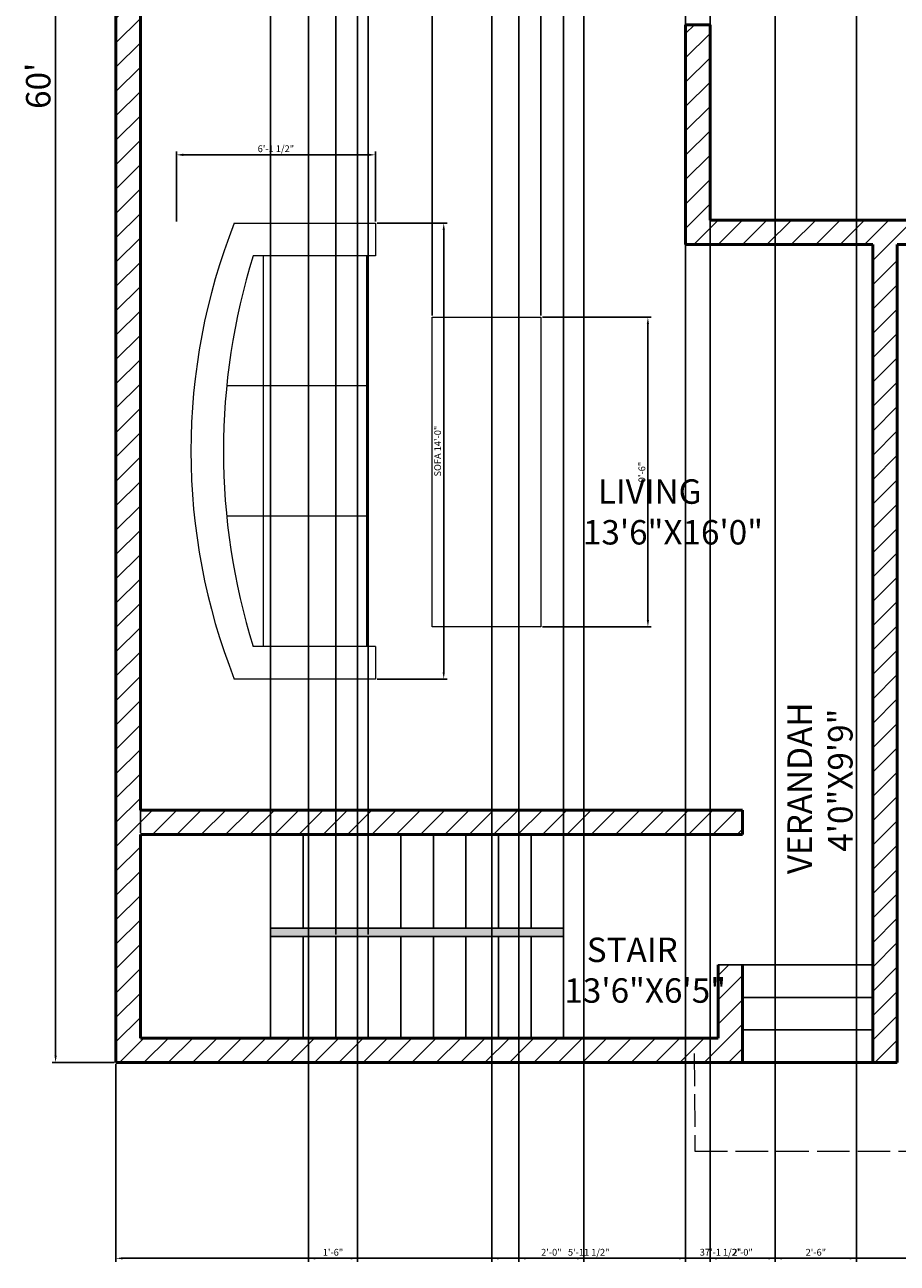
# Model space of a CAD drawing. Units: inches. Extents: x 2758 to 3288, y 1211 to 2050.
# Tile 1 of 4: x 2768 to 3089, y 1211 to 1667. Entities that reach past the tile are written whole.
import ezdxf

# ---------------------------------------------------------------- set-up
doc = ezdxf.new("R2010")
doc.units = ezdxf.units.IN
doc.linetypes.add('ACAD_ISO02W100', pattern=[15, 12, -3])
for name, color, linetype, lineweight in [('A-ANNO-DIMS', 2, 'Continuous', 18), ('A-AREA-IDEN', 7, 'Continuous', 25), ('A-FLOR-STRS', 7, 'Continuous', 25), ('A-FURN', 8, 'Continuous', 18), ('A-WALL', 7, 'Continuous', 50)]:
    doc.layers.add(name, color=color, linetype=linetype, lineweight=lineweight)
for name, color, linetype, lineweight, true_color in [('A-FLOR-OVHD', 244, 'ACAD_ISO02W100', 18, 0x991b1e), ('A-FLOR-PATT', 244, 'Continuous', 13, 0x991b1e), ('A-WALL-PATT', 244, 'Continuous', 13, 0x991b1e)]:
    doc.layers.add(name, color=color, linetype=linetype, lineweight=lineweight, true_color=true_color)
doc.styles.get("Standard").update_dxf_attribs({"font": 'arial.ttf'})
doc.dimstyles.new('ISO-25', dxfattribs={"dimtxt": 2.5, "dimasz": 2.5, "dimexe": 1.25, "dimexo": 0.625, "dimtad": 1, "dimlunit": 3, "dimtxsty": 'Standard', "dimcen": 2.5, "dimadec": 0, "dimazin": 0, "dimtfac": 1, "dimtmove": 0, "dimatfit": 3, "dimfxl": 1, "dimarcsym": 0})

# ---------------------------------------------------------------- blocks, each defined once
blk = doc.blocks.new('Sofa - Roundback 7 ft.')
for p, q in [((-12.00002, -32.4421), (-12.00003, -6.5971)), ((11.99997, -32.4421), (11.99998, -6.5971)), ((-36.000027, -34), (-36.000027, -11.4696)), ((-35.999844, -13.3819), (35.9998, -13.3819)), ((35.99998, -34), (35.99998, -11.4696)), ((-36.000027, -32.4421), (35.99998, -32.4421))]:
    blk.add_line(p, q)
for points in [[(-36.000027, -34), (-42.000027, -34), (-42.000027, -8)], [(41.99998, -8), (41.99998, -34), (35.99998, -34)]]:
    blk.add_lwpolyline(points)
for centre, radius, start, end in [((0, -114.25), 114.25, 68.43141, 111.5686), ((-0.00001, -127.1968), 121.1968, 72.72033, 107.2797)]:
    blk.add_arc(centre, radius, start, end)
blk = doc.blocks.new('*D7')
at = {"layer": 'A-ANNO-DIMS', "color": 0, "lineweight": -2, "transparency": 16777216}
for p, q in [((2801.18, 2004.81), (2777.63, 2004.81)), ((2778.88, 2002.31), (2778.88, 1287.31)), ((2800.51, 1284.81), (2777.63, 1284.81))]:
    blk.add_line(p, q, dxfattribs=at)
at = {"layer": 'A-ANNO-DIMS', "color": 0, "transparency": 16777216}
for points in [[(2778.47, 2002.31), (2779.3, 2002.31), (2778.88, 2004.81)], [(2778.47, 1287.31), (2779.3, 1287.31), (2778.88, 1284.81)]]:
    blk.add_solid(points, dxfattribs=at)
at = {"layer": 'Defpoints', "color": 0, "transparency": 16777216}
for p in [(2801.81, 2004.81), (2778.88, 1284.81), (2801.14, 1284.81)]:
    blk.add_point(p, dxfattribs=at)
at = {"layer": 'A-ANNO-DIMS', "color": 0, "transparency": 16777216, "insert": (2773.66, 1644.81), "char_height": 9, "attachment_point": 5, "rotation": 90}
blk.add_mtext("60'", dxfattribs=at)
blk = doc.blocks.new('*D16')
at = {"layer": 'A-ANNO-DIMS', "color": 0, "lineweight": -2, "transparency": 16777216}
for p, q in [((2897.39, 1594.17), (2923.22, 1594.17)), ((2921.97, 1428.67), (2921.97, 1591.67)), ((2897.39, 1426.17), (2923.22, 1426.17))]:
    blk.add_line(p, q, dxfattribs=at)
at = {"layer": 'A-ANNO-DIMS', "color": 0, "transparency": 16777216}
for points in [[(2921.55, 1591.67), (2922.39, 1591.67), (2921.97, 1594.17)], [(2921.55, 1428.67), (2922.39, 1428.67), (2921.97, 1426.17)]]:
    blk.add_solid(points, dxfattribs=at)
at = {"layer": 'Defpoints', "color": 0, "transparency": 16777216}
for p in [(2896.77, 1594.17), (2921.97, 1594.17), (2896.77, 1426.17)]:
    blk.add_point(p, dxfattribs=at)
at = {"layer": 'A-ANNO-DIMS', "color": 0, "transparency": 16777216, "insert": (2920.05, 1510.17), "char_height": 2.5, "attachment_point": 5, "rotation": 90}
blk.add_mtext('SOFA 14\'-0"', dxfattribs=at)
blk = doc.blocks.new('*D17')
at = {"layer": 'A-ANNO-DIMS', "color": 0, "lineweight": -2, "transparency": 16777216}
for p, q in [((2823.44, 1594.8), (2823.44, 1620.62)), ((2896.77, 1594.8), (2896.77, 1620.62)), ((2894.27, 1619.37), (2825.94, 1619.37))]:
    blk.add_line(p, q, dxfattribs=at)
at = {"layer": 'A-ANNO-DIMS', "color": 0, "transparency": 16777216}
for points in [[(2825.94, 1619.79), (2825.94, 1618.95), (2823.44, 1619.37)], [(2894.27, 1619.79), (2894.27, 1618.95), (2896.77, 1619.37)]]:
    blk.add_solid(points, dxfattribs=at)
at = {"layer": 'Defpoints', "color": 0, "transparency": 16777216}
for p in [(2823.44, 1619.37), (2823.44, 1594.17), (2896.77, 1594.17)]:
    blk.add_point(p, dxfattribs=at)
at = {"layer": 'A-ANNO-DIMS', "color": 0, "transparency": 16777216, "insert": (2860.1, 1621.29), "char_height": 2.5, "attachment_point": 5}
blk.add_mtext('6\'-1 1/2"', dxfattribs=at)
blk = doc.blocks.new('*D18')
at = {"layer": 'A-ANNO-DIMS', "color": 0, "lineweight": -2, "transparency": 16777216}
for p, q in [((2801.14, 1284.19), (2801.14, 1211.4)), ((3246.84, 1251.47), (3246.84, 1211.4)), ((2803.64, 1212.65), (3244.34, 1212.65))]:
    blk.add_line(p, q, dxfattribs=at)
at = {"layer": 'A-ANNO-DIMS', "color": 0, "transparency": 16777216}
for points in [[(2803.64, 1213.06), (2803.64, 1212.23), (2801.14, 1212.65)], [(3244.34, 1213.06), (3244.34, 1212.23), (3246.84, 1212.65)]]:
    blk.add_solid(points, dxfattribs=at)
at = {"layer": 'Defpoints', "color": 0, "transparency": 16777216}
for p in [(2801.14, 1284.81), (3246.84, 1252.1), (3246.84, 1212.65)]:
    blk.add_point(p, dxfattribs=at)
at = {"layer": 'A-ANNO-DIMS', "color": 0, "transparency": 16777216, "insert": (3023.99, 1214.57), "char_height": 2.5, "attachment_point": 5}
blk.add_mtext('37\'-1 1/2"', dxfattribs=at)
blk = doc.blocks.new('*D24')
at = {"layer": 'A-ANNO-DIMS', "color": 0, "lineweight": -2, "transparency": 16777216}
for p, q in [((2872.14, 1920.19), (2872.14, 1211.4)), ((2890.14, 1920.19), (2890.14, 1211.4)), ((2874.64, 1212.65), (2887.64, 1212.65))]:
    blk.add_line(p, q, dxfattribs=at)
at = {"layer": 'A-ANNO-DIMS', "color": 0, "transparency": 16777216}
for points in [[(2874.64, 1213.06), (2874.64, 1212.23), (2872.14, 1212.65)], [(2887.64, 1213.06), (2887.64, 1212.23), (2890.14, 1212.65)]]:
    blk.add_solid(points, dxfattribs=at)
at = {"layer": 'Defpoints', "color": 0, "transparency": 16777216}
for p in [(2872.14, 1920.81), (2890.14, 1920.81), (2890.14, 1212.65)]:
    blk.add_point(p, dxfattribs=at)
at = {"layer": 'A-ANNO-DIMS', "color": 0, "transparency": 16777216, "insert": (2881.14, 1214.55), "char_height": 2.5, "attachment_point": 5}
blk.add_mtext('1\'-6"', dxfattribs=at)
blk = doc.blocks.new('*D27')
at = {"layer": 'A-ANNO-DIMS', "color": 0, "lineweight": -2, "transparency": 16777216}
for p, q in [((3044.14, 1723.69), (3044.14, 1211.4)), ((3074.14, 1723.69), (3074.14, 1211.4)), ((3046.64, 1212.65), (3071.64, 1212.65))]:
    blk.add_line(p, q, dxfattribs=at)
at = {"layer": 'A-ANNO-DIMS', "color": 0, "transparency": 16777216}
for points in [[(3046.64, 1213.06), (3046.64, 1212.23), (3044.14, 1212.65)], [(3071.64, 1213.06), (3071.64, 1212.23), (3074.14, 1212.65)]]:
    blk.add_solid(points, dxfattribs=at)
at = {"layer": 'Defpoints', "color": 0, "transparency": 16777216}
for p in [(3044.14, 1724.31), (3074.14, 1724.31), (3074.14, 1212.65)]:
    blk.add_point(p, dxfattribs=at)
at = {"layer": 'A-ANNO-DIMS', "color": 0, "transparency": 16777216, "insert": (3059.14, 1214.55), "char_height": 2.5, "attachment_point": 5}
blk.add_mtext('2\'-6"', dxfattribs=at)
blk = doc.blocks.new('*D28')
at = {"layer": 'A-ANNO-DIMS', "color": 0, "lineweight": -2, "transparency": 16777216}
for p, q in [((2939.69, 1723.69), (2939.69, 1211.4)), ((3011.14, 1723.69), (3011.14, 1211.4)), ((2942.19, 1212.65), (3008.64, 1212.65))]:
    blk.add_line(p, q, dxfattribs=at)
at = {"layer": 'A-ANNO-DIMS', "color": 0, "transparency": 16777216}
for points in [[(2942.19, 1213.06), (2942.19, 1212.23), (2939.69, 1212.65)], [(3008.64, 1213.06), (3008.64, 1212.23), (3011.14, 1212.65)]]:
    blk.add_solid(points, dxfattribs=at)
at = {"layer": 'Defpoints', "color": 0, "transparency": 16777216}
for p in [(2939.69, 1724.31), (3011.14, 1724.31), (3011.14, 1212.65)]:
    blk.add_point(p, dxfattribs=at)
at = {"layer": 'A-ANNO-DIMS', "color": 0, "transparency": 16777216, "insert": (2975.42, 1214.56), "char_height": 2.5, "attachment_point": 5}
blk.add_mtext('5\'-11 1/2"', dxfattribs=at)
blk = doc.blocks.new('*D29')
at = {"layer": 'A-ANNO-DIMS', "color": 0, "lineweight": -2, "transparency": 16777216}
for p, q in [((2858.14, 1369.44), (2858.14, 2045.51)), ((2966.14, 1369.44), (2966.14, 2045.51)), ((2860.64, 2044.26), (2963.64, 2044.26))]:
    blk.add_line(p, q, dxfattribs=at)
at = {"layer": 'A-ANNO-DIMS', "color": 0, "transparency": 16777216}
for points in [[(2860.64, 2044.68), (2860.64, 2043.84), (2858.14, 2044.26)], [(2963.64, 2044.68), (2963.64, 2043.84), (2966.14, 2044.26)]]:
    blk.add_solid(points, dxfattribs=at)
at = {"layer": 'Defpoints', "color": 0, "transparency": 16777216}
for p in [(2966.14, 2044.26), (2858.14, 1368.81), (2966.14, 1368.81)]:
    blk.add_point(p, dxfattribs=at)
at = {"layer": 'A-ANNO-DIMS', "color": 0, "transparency": 16777216, "insert": (2912.14, 2046.16), "char_height": 2.5, "attachment_point": 5}
blk.add_mtext('9\'-0"', dxfattribs=at)
blk = doc.blocks.new('*D30')
at = {"layer": 'A-ANNO-DIMS', "color": 0, "lineweight": -2, "transparency": 16777216}
for p, q in [((2882.14, 1331.94), (2882.14, 2045.51)), ((2894.14, 1331.94), (2894.14, 2045.51)), ((2884.64, 2044.26), (2891.64, 2044.26))]:
    blk.add_line(p, q, dxfattribs=at)
at = {"layer": 'A-ANNO-DIMS', "color": 0, "transparency": 16777216}
for points in [[(2884.64, 2044.68), (2884.64, 2043.84), (2882.14, 2044.26)], [(2891.64, 2044.68), (2891.64, 2043.84), (2894.14, 2044.26)]]:
    blk.add_solid(points, dxfattribs=at)
at = {"layer": 'Defpoints', "color": 0, "transparency": 16777216}
for p in [(2894.14, 2044.26), (2882.14, 1331.31), (2894.14, 1331.31)]:
    blk.add_point(p, dxfattribs=at)
at = {"layer": 'A-ANNO-DIMS', "color": 0, "transparency": 16777216, "insert": (2888.14, 2046.16), "char_height": 2.5, "attachment_point": 5}
blk.add_mtext('1\'-0"', dxfattribs=at)
blk = doc.blocks.new('*D31')
at = {"layer": 'A-ANNO-DIMS', "color": 0, "lineweight": -2, "transparency": 16777216}
for p, q in [((2810.14, 1369.44), (2810.14, 2045.51)), ((2858.14, 1369.44), (2858.14, 2045.51)), ((2812.64, 2044.26), (2855.64, 2044.26))]:
    blk.add_line(p, q, dxfattribs=at)
at = {"layer": 'A-ANNO-DIMS', "color": 0, "transparency": 16777216}
for points in [[(2812.64, 2044.68), (2812.64, 2043.84), (2810.14, 2044.26)], [(2855.64, 2044.68), (2855.64, 2043.84), (2858.14, 2044.26)]]:
    blk.add_solid(points, dxfattribs=at)
at = {"layer": 'Defpoints', "color": 0, "transparency": 16777216}
for p in [(2858.14, 2044.26), (2810.14, 1368.81), (2858.14, 1368.81)]:
    blk.add_point(p, dxfattribs=at)
at = {"layer": 'A-ANNO-DIMS', "color": 0, "transparency": 16777216, "insert": (2834.14, 2046.16), "char_height": 2.5, "attachment_point": 5}
blk.add_mtext('4\'-0"', dxfattribs=at)
blk = doc.blocks.new('*D32')
at = {"layer": 'A-ANNO-DIMS', "color": 0, "lineweight": -2, "transparency": 16777216}
for p, q in [((2949.64, 1840.69), (2949.64, 1211.4)), ((2973.64, 1840.69), (2973.64, 1211.4)), ((2952.14, 1212.65), (2971.14, 1212.65))]:
    blk.add_line(p, q, dxfattribs=at)
at = {"layer": 'A-ANNO-DIMS', "color": 0, "transparency": 16777216}
for points in [[(2952.14, 1213.06), (2952.14, 1212.23), (2949.64, 1212.65)], [(2971.14, 1213.06), (2971.14, 1212.23), (2973.64, 1212.65)]]:
    blk.add_solid(points, dxfattribs=at)
at = {"layer": 'Defpoints', "color": 0, "transparency": 16777216}
for p in [(2949.64, 1841.31), (2973.64, 1841.31), (2973.64, 1212.65)]:
    blk.add_point(p, dxfattribs=at)
at = {"layer": 'A-ANNO-DIMS', "color": 0, "transparency": 16777216, "insert": (2961.64, 1214.55), "char_height": 2.5, "attachment_point": 5}
blk.add_mtext('2\'-0"', dxfattribs=at)
blk = doc.blocks.new('*D35')
at = {"layer": 'A-ANNO-DIMS', "color": 0, "lineweight": -2, "transparency": 16777216}
for p, q in [((2917.71, 1560.11), (2917.71, 2045.51)), ((2957.78, 1560.11), (2957.78, 2045.51)), ((2920.21, 2044.26), (2955.28, 2044.26))]:
    blk.add_line(p, q, dxfattribs=at)
at = {"layer": 'A-ANNO-DIMS', "color": 0, "transparency": 16777216}
for points in [[(2920.21, 2044.68), (2920.21, 2043.84), (2917.71, 2044.26)], [(2955.28, 2044.68), (2955.28, 2043.84), (2957.78, 2044.26)]]:
    blk.add_solid(points, dxfattribs=at)
at = {"layer": 'Defpoints', "color": 0, "transparency": 16777216}
for p in [(2957.78, 2044.26), (2917.71, 1559.49), (2957.78, 1559.49)]:
    blk.add_point(p, dxfattribs=at)
at = {"layer": 'A-ANNO-DIMS', "color": 0, "transparency": 16777216, "insert": (2937.75, 2046.16), "char_height": 2.5, "attachment_point": 5}
blk.add_mtext('3\'-4"', dxfattribs=at)
blk = doc.blocks.new('*D36')
at = {"layer": 'A-ANNO-DIMS', "color": 0, "lineweight": -2, "transparency": 16777216}
for p, q in [((2958.41, 1559.49), (2998.48, 1559.49)), ((2997.23, 1556.99), (2997.23, 1447.93)), ((2958.41, 1445.43), (2998.48, 1445.43))]:
    blk.add_line(p, q, dxfattribs=at)
at = {"layer": 'A-ANNO-DIMS', "color": 0, "transparency": 16777216}
for points in [[(2996.82, 1556.99), (2997.65, 1556.99), (2997.23, 1559.49)], [(2996.82, 1447.93), (2997.65, 1447.93), (2997.23, 1445.43)]]:
    blk.add_solid(points, dxfattribs=at)
at = {"layer": 'Defpoints', "color": 0, "transparency": 16777216}
for p in [(2957.78, 1559.49), (2957.78, 1445.43), (2997.23, 1445.43)]:
    blk.add_point(p, dxfattribs=at)
at = {"layer": 'A-ANNO-DIMS', "color": 0, "transparency": 16777216, "insert": (2995.33, 1502.46), "char_height": 2.5, "attachment_point": 5, "rotation": 90}
blk.add_mtext('9\'-6"', dxfattribs=at)
blk = doc.blocks.new('*D37')
at = {"layer": 'A-ANNO-DIMS', "color": 0, "lineweight": -2, "transparency": 16777216}
for p, q in [((3020.14, 1714.69), (3020.14, 1211.4)), ((3044.14, 1714.69), (3044.14, 1211.4)), ((3022.64, 1212.65), (3041.64, 1212.65))]:
    blk.add_line(p, q, dxfattribs=at)
at = {"layer": 'A-ANNO-DIMS', "color": 0, "transparency": 16777216}
for points in [[(3022.64, 1213.06), (3022.64, 1212.23), (3020.14, 1212.65)], [(3041.64, 1213.06), (3041.64, 1212.23), (3044.14, 1212.65)]]:
    blk.add_solid(points, dxfattribs=at)
at = {"layer": 'Defpoints', "color": 0, "transparency": 16777216}
for p in [(3020.14, 1715.31), (3044.14, 1715.31), (3044.14, 1212.65)]:
    blk.add_point(p, dxfattribs=at)
at = {"layer": 'A-ANNO-DIMS', "color": 0, "transparency": 16777216, "insert": (3032.14, 1214.55), "char_height": 2.5, "attachment_point": 5}
blk.add_mtext('2\'-0"', dxfattribs=at)

msp = doc.modelspace()

# ---------------------------------------------------------------- hatches: boundary and pattern name
at = {"layer": 'A-FLOR-PATT'}
h = msp.add_hatch(color=256, dxfattribs=at)
h.dxf.hatch_style = 1
h.paths.add_polyline_path([(2966.139, 1334.31), (2858.139, 1334.31), (2858.139, 1331.31), (2966.139, 1331.31)])
at = {"layer": 'A-WALL-PATT'}
h = msp.add_hatch(dxfattribs=at)
h.set_pattern_fill('ANSI31', color=256, scale=2)
h.paths.add_polyline_path([(2810.139, 1377.81), (2810.139, 1715.31), (2939.691, 1715.31), (2939.691, 1724.31), (2910.639, 1724.31), (2910.639, 1778.31), (2906.139, 1778.31), (2906.139, 1724.31), (2896.389, 1724.31), (2810.139, 1724.31), (2810.139, 1796.31), (2982.639, 1796.31), (2982.639, 1800.81), (2810.139, 1800.81), (2810.139, 1920.81), (2872.139, 1920.81), (2872.139, 1929.81), (2810.139, 1929.81), (2810.139, 1995.81), (2890.139, 1995.81), (2890.139, 1920.81), (2973.639, 1920.81), (2973.639, 1841.31), (2949.639, 1841.31), (2949.639, 1836.81), (2973.639, 1836.81), (3114.639, 1836.81), (3114.639, 1887.81), (3110.139, 1887.81), (3110.139, 1845.81), (2982.639, 1845.81), (2982.639, 1977.81), (2973.639, 1977.81), (2973.639, 1929.81), (2894.639, 1929.81), (2894.639, 1995.81), (3152.139, 1995.81), (3152.139, 1800.81), (3152.139, 1796.31), (3152.139, 1724.31), (3074.139, 1724.31), (3074.139, 1715.31), (3152.139, 1715.31), (3152.139, 1595.31), (3020.139, 1595.31), (3020.139, 1667.31), (3011.139, 1667.31), (3011.139, 1586.31), (3080.139, 1586.31), (3080.139, 1284.81), (3089.139, 1284.81), (3089.139, 1586.31), (3161.139, 1586.31), (3161.139, 2004.81), (2801.139, 2004.81), (2801.139, 1284.81), (3032.139, 1284.81), (3032.139, 1320.81), (3023.139, 1320.81), (3023.139, 1293.81), (2810.139, 1293.81), (2810.139, 1368.81), (3032.139, 1368.81), (3032.139, 1377.81)])

# ---------------------------------------------------------------- linework, layer by layer
at = {"layer": 'A-FLOR-OVHD'}
for p, q in [((3014.24, 1288.096), (3014.57, 1252.097)), ((3014.57, 1252.097), (3246.836, 1252.097))]:
    msp.add_line(p, q, dxfattribs=at)
at = {"layer": 'A-FLOR-STRS'}
for p, q in [((2858.139, 1293.81), (2858.139, 1368.81)), ((2870.139, 1334.31), (2870.139, 1368.81)), ((2882.139, 1334.31), (2882.139, 1368.81)), ((2894.139, 1334.31), (2894.139, 1368.81)), ((2906.139, 1334.31), (2906.139, 1368.81)), ((2918.139, 1334.31), (2918.139, 1368.81)), ((2930.139, 1334.31), (2930.139, 1368.81)), ((2942.139, 1334.31), (2942.139, 1368.81)), ((2954.139, 1334.31), (2954.139, 1368.81)), ((2966.139, 1293.81), (2966.139, 1368.81)), ((2858.139, 1334.31), (2966.139, 1334.31)), ((2858.139, 1331.31), (2966.139, 1331.31)), ((2870.139, 1293.81), (2870.139, 1331.31)), ((2882.139, 1293.81), (2882.139, 1331.31)), ((2894.139, 1293.81), (2894.139, 1331.31)), ((2906.139, 1293.81), (2906.139, 1331.31)), ((2918.139, 1293.81), (2918.139, 1331.31)), ((2930.139, 1293.81), (2930.139, 1331.31)), ((2942.139, 1293.81), (2942.139, 1331.31)), ((2954.139, 1293.81), (2954.139, 1331.31)), ((3080.139, 1320.81), (3023.139, 1320.81)), ((3080.139, 1308.81), (3032.139, 1308.81)), ((3080.139, 1308.81), (3032.139, 1308.81)), ((3080.139, 1296.81), (3032.139, 1296.81))]:
    msp.add_line(p, q, dxfattribs=at)
at = {"layer": 'A-FURN'}
msp.add_lwpolyline([(2917.71, 1559.489), (2957.785, 1559.489), (2957.785, 1445.432), (2917.71, 1445.432)], close=True, dxfattribs=at)
at = {"layer": 'A-WALL'}
for p, q in [((2801.139, 1284.81), (2801.139, 2004.81)), ((2810.139, 1523.31), (2810.139, 1715.31)), ((3011.139, 1667.31), (3020.139, 1667.31)), ((3011.139, 1667.31), (3011.139, 1586.31)), ((3020.139, 1667.31), (3020.139, 1595.31)), ((3020.139, 1595.31), (3152.139, 1595.31)), ((3011.139, 1586.31), (3080.139, 1586.31)), ((3080.139, 1284.81), (3080.139, 1586.31)), ((3089.139, 1284.81), (3089.139, 1586.31)), ((3089.139, 1586.31), (3161.139, 1586.31)), ((2810.139, 1377.81), (2810.139, 1523.31)), ((3032.139, 1377.81), (2810.139, 1377.81)), ((3032.139, 1368.81), (3032.139, 1377.81)), ((2810.139, 1293.81), (2810.139, 1368.81)), ((3032.139, 1368.81), (2810.139, 1368.81)), ((3023.139, 1293.81), (3023.139, 1320.81)), ((3032.139, 1284.81), (3032.139, 1320.81)), ((3023.139, 1293.81), (2810.139, 1293.81)), ((3089.139, 1284.81), (2801.139, 1284.81)), ((3089.139, 1284.81), (2801.139, 1284.81))]:
    msp.add_line(p, q, dxfattribs=at)

# ---------------------------------------------------------------- block references
at = {"layer": 'A-FURN', "xscale": 2, "yscale": 2, "zscale": 2, "rotation": 90}
msp.add_blockref('Sofa - Roundback 7 ft.', (2828.77, 1510.171), dxfattribs=at)

# ---------------------------------------------------------------- texts
at = {"layer": 'A-AREA-IDEN', "char_height": 9, "attachment_point": 1}
for s, insert in [('  LIVING\\P13\'6"X16\'0"', (2973.263, 1499.754)), ('   STAIR\\P13\'6"X6\'5"', (2966.439, 1330.851))]:
    msp.add_mtext_dynamic_manual_height_columns(s, width=130.32194, gutter_width=12.5, heights=[77.844], dxfattribs=dict(at, insert=insert))
at = {"layer": 'A-AREA-IDEN', "insert": (3048.671, 1354.247), "char_height": 9, "attachment_point": 1, "rotation": 90}
msp.add_mtext_dynamic_manual_height_columns('VERANDAH\\P   4\'0"X9\'9"', width=130.32194, gutter_width=12.5, heights=[77.844], dxfattribs=at)

# ---------------------------------------------------------------- dimensions: what is measured, and where the dimension line sits
at = {"layer": 'A-ANNO-DIMS'}
for base, p1, p2, picture, middle in [((2858.139, 2044.26), (2810.139, 1368.81), (2858.139, 1368.81), '*D31', (2834.139, 2046.162)), ((2966.139, 2044.26), (2858.139, 1368.81), (2966.139, 1368.81), '*D29', (2912.139, 2046.162)), ((2894.139, 2044.26), (2882.139, 1331.31), (2894.139, 1331.31), '*D30', (2888.139, 2046.162)), ((2957.785, 2044.26), (2917.71, 1559.489), (2957.785, 1559.489), '*D35', (2937.747, 2046.163)), ((2890.139, 1212.647), (2872.139, 1920.81), (2890.139, 1920.81), '*D24', (2881.139, 1214.549)), ((2973.639, 1212.647), (2949.639, 1841.31), (2973.639, 1841.31), '*D32', (2961.639, 1214.549)), ((3011.139, 1212.647), (2939.691, 1724.31), (3011.139, 1724.31), '*D28', (2975.415, 1214.565)), ((3074.139, 1212.647), (3044.139, 1724.31), (3074.139, 1724.31), '*D27', (3059.139, 1214.549)), ((3044.139, 1212.647), (3020.139, 1715.31), (3044.139, 1715.31), '*D37', (3032.139, 1214.549)), ((3246.836, 1212.647), (2801.139, 1284.81), (3246.836, 1252.097), '*D18', (3023.987, 1214.566))]:
    dim = msp.add_linear_dim(base=base, p1=p1, p2=p2, dimstyle='ISO-25', override={"dimdec": 1, "dimlfac": 1, "dimrnd": 0, "dimzin": 1, "dimdsep": 46, "dimlunit": 4, "dimfrac": 2}, dxfattribs=at)
    dim.commit()
    dim.dimension.update_dxf_attribs({"geometry": picture, "text_midpoint": middle})
for base, p1, p2, angle, override, picture, middle in [((2778.882, 1284.81), (2801.807, 2004.81), (2801.139, 1284.81), 90, {"dimtxt": 9, "dimclrd": 0, "dimclre": 0, "dimclrt": 0}, '*D7', (2773.662, 1644.81)), ((2823.436, 1619.371), (2896.77, 1594.171), (2823.436, 1594.171), 180, {"dimdec": 1, "dimlfac": 1, "dimrnd": 0, "dimzin": 1, "dimdsep": 46, "dimlunit": 4, "dimfrac": 2}, '*D17', (2860.103, 1621.288)), ((2997.235, 1445.432), (2957.785, 1559.489), (2957.785, 1445.432), 270, {"dimdec": 1, "dimlfac": 1, "dimrnd": 0, "dimzin": 1, "dimdsep": 46, "dimlunit": 4, "dimfrac": 2}, '*D36', (2995.333, 1502.46))]:
    dim = msp.add_linear_dim(base=base, p1=p1, p2=p2, angle=angle, dimstyle='ISO-25', override=override, dxfattribs=at)
    dim.commit()
    dim.dimension.update_dxf_attribs({"geometry": picture, "text_midpoint": middle})
dim = msp.add_linear_dim(base=(2921.97, 1594.171), p1=(2896.77, 1426.17), p2=(2896.77, 1594.171), angle=90, text='SOFA <>', dimstyle='ISO-25', override={"dimdec": 1, "dimlfac": 1, "dimrnd": 0, "dimzin": 1, "dimdsep": 46, "dimlunit": 4, "dimfrac": 2}, dxfattribs=at)
dim.commit()
dim.dimension.update_dxf_attribs({"geometry": '*D16', "text_midpoint": (2920.051, 1510.17)})

doc.saveas('drawing.dxf')
